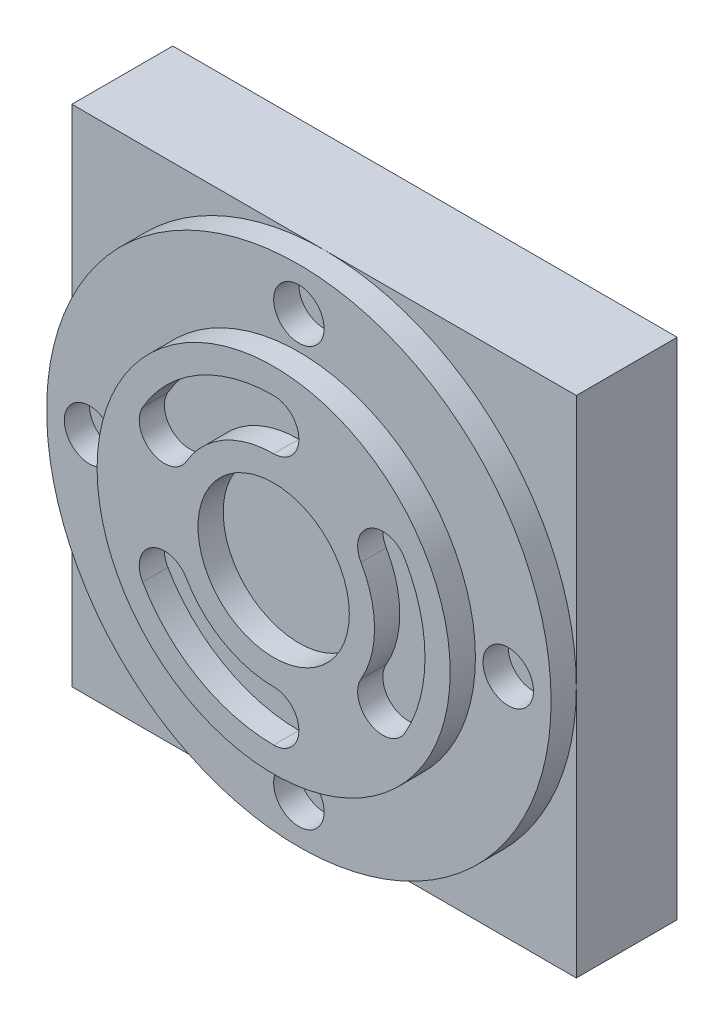
ISO-10303-21;
HEADER;
FILE_DESCRIPTION(('STEP AP214'),'2;1');
FILE_NAME('part.step','',(''),(''),'','','');
FILE_SCHEMA(('AUTOMOTIVE_DESIGN { 1 0 10303 214 1 1 1 1 }'));
ENDSEC;
DATA;
#1=APPLICATION_CONTEXT('core data for automotive mechanical design processes');
#2=APPLICATION_PROTOCOL_DEFINITION('international standard','automotive_design',2000,#1);
#3=PRODUCT_CONTEXT('',#1,'mechanical');
#4=PRODUCT('Part','Part','',(#3));
#5=PRODUCT_RELATED_PRODUCT_CATEGORY('part','',(#4));
#6=PRODUCT_DEFINITION_FORMATION('','',#4);
#7=PRODUCT_DEFINITION_CONTEXT('part definition',#1,'design');
#8=PRODUCT_DEFINITION('design','',#6,#7);
#9=PRODUCT_DEFINITION_SHAPE('','',#8);
#10=(LENGTH_UNIT() NAMED_UNIT(*) SI_UNIT(.MILLI.,.METRE.));
#11=(NAMED_UNIT(*) PLANE_ANGLE_UNIT() SI_UNIT($,.RADIAN.));
#12=(NAMED_UNIT(*) SI_UNIT($,.STERADIAN.) SOLID_ANGLE_UNIT());
#13=UNCERTAINTY_MEASURE_WITH_UNIT(LENGTH_MEASURE(1.E-05),#10,'distance_accuracy_value','');
#14=(GEOMETRIC_REPRESENTATION_CONTEXT(3) GLOBAL_UNCERTAINTY_ASSIGNED_CONTEXT((#13)) GLOBAL_UNIT_ASSIGNED_CONTEXT((#10,
#11,#12)) REPRESENTATION_CONTEXT('',''));
#15=CARTESIAN_POINT('',(0.,0.,0.));
#16=DIRECTION('',(0.,0.,1.));
#17=DIRECTION('',(1.,0.,0.));
#18=AXIS2_PLACEMENT_3D('',#15,#16,#17);
#19=CARTESIAN_POINT('',(0.,0.,20.));
#20=DIRECTION('',(0.,0.,1.));
#21=DIRECTION('',(1.,0.,0.));
#22=AXIS2_PLACEMENT_3D('',#19,#20,#21);
#23=PLANE('',#22);
#24=CARTESIAN_POINT('',(50.,50.,20.));
#25=DIRECTION('',(0.,0.,1.));
#26=DIRECTION('',(1.,0.,0.));
#27=AXIS2_PLACEMENT_3D('',#24,#25,#26);
#28=CIRCLE('',#27,50.);
#29=CARTESIAN_POINT('',(100.,50.,20.));
#30=VERTEX_POINT('',#29);
#31=CARTESIAN_POINT('',(50.,100.,20.));
#32=VERTEX_POINT('',#31);
#33=EDGE_CURVE('E49',#30,#32,#28,.T.);
#34=ORIENTED_EDGE('',*,*,#33,.F.);
#35=DIRECTION('',(0.,1.,0.));
#36=VECTOR('',#35,1.);
#37=CARTESIAN_POINT('',(100.,0.,20.));
#38=LINE('',#37,#36);
#39=CARTESIAN_POINT('',(100.,100.,20.));
#40=VERTEX_POINT('',#39);
#41=EDGE_CURVE('E320',#30,#40,#38,.T.);
#42=ORIENTED_EDGE('',*,*,#41,.T.);
#43=DIRECTION('',(-1.,0.,0.));
#44=VECTOR('',#43,1.);
#45=CARTESIAN_POINT('',(100.,100.,20.));
#46=LINE('',#45,#44);
#47=EDGE_CURVE('E321',#40,#32,#46,.T.);
#48=ORIENTED_EDGE('',*,*,#47,.T.);
#49=EDGE_LOOP('',(#34,#42,#48));
#50=FACE_BOUND('',#49,.T.);
#51=ADVANCED_FACE('F39',(#50),#23,.T.);
#52=CARTESIAN_POINT('',(0.,50.,20.));
#53=VERTEX_POINT('',#52);
#54=EDGE_CURVE('E11',#32,#53,#28,.T.);
#55=ORIENTED_EDGE('',*,*,#54,.F.);
#56=CARTESIAN_POINT('',(0.,100.,20.));
#57=VERTEX_POINT('',#56);
#58=EDGE_CURVE('E319',#32,#57,#46,.T.);
#59=ORIENTED_EDGE('',*,*,#58,.T.);
#60=DIRECTION('',(0.,-1.,0.));
#61=VECTOR('',#60,1.);
#62=CARTESIAN_POINT('',(0.,100.,20.));
#63=LINE('',#62,#61);
#64=EDGE_CURVE('E310',#57,#53,#63,.T.);
#65=ORIENTED_EDGE('',*,*,#64,.T.);
#66=EDGE_LOOP('',(#55,#59,#65));
#67=FACE_BOUND('',#66,.T.);
#68=ADVANCED_FACE('F360',(#67),#23,.T.);
#69=CARTESIAN_POINT('',(50.,0.,20.));
#70=VERTEX_POINT('',#69);
#71=EDGE_CURVE('E48',#53,#70,#28,.T.);
#72=ORIENTED_EDGE('',*,*,#71,.F.);
#73=CARTESIAN_POINT('',(0.,0.,20.));
#74=VERTEX_POINT('',#73);
#75=EDGE_CURVE('E311',#53,#74,#63,.T.);
#76=ORIENTED_EDGE('',*,*,#75,.T.);
#77=DIRECTION('',(1.,0.,0.));
#78=VECTOR('',#77,1.);
#79=CARTESIAN_POINT('',(0.,0.,20.));
#80=LINE('',#79,#78);
#81=EDGE_CURVE('E314',#74,#70,#80,.T.);
#82=ORIENTED_EDGE('',*,*,#81,.T.);
#83=EDGE_LOOP('',(#72,#76,#82));
#84=FACE_BOUND('',#83,.T.);
#85=ADVANCED_FACE('F355',(#84),#23,.T.);
#86=CARTESIAN_POINT('',(0.,100.,20.));
#87=DIRECTION('',(1.,0.,0.));
#88=DIRECTION('',(0.,0.,-1.));
#89=AXIS2_PLACEMENT_3D('',#86,#87,#88);
#90=PLANE('',#89);
#91=DIRECTION('',(0.,-1.,0.));
#92=VECTOR('',#91,1.);
#93=CARTESIAN_POINT('',(0.,100.,0.));
#94=LINE('',#93,#92);
#95=CARTESIAN_POINT('',(0.,100.,0.));
#96=VERTEX_POINT('',#95);
#97=CARTESIAN_POINT('',(0.,0.,0.));
#98=VERTEX_POINT('',#97);
#99=EDGE_CURVE('E304',#96,#98,#94,.T.);
#100=ORIENTED_EDGE('',*,*,#99,.T.);
#101=DIRECTION('',(0.,0.,-1.));
#102=VECTOR('',#101,1.);
#103=CARTESIAN_POINT('',(0.,0.,20.));
#104=LINE('',#103,#102);
#105=EDGE_CURVE('E43',#74,#98,#104,.T.);
#106=ORIENTED_EDGE('',*,*,#105,.F.);
#107=ORIENTED_EDGE('',*,*,#75,.F.);
#108=ORIENTED_EDGE('',*,*,#64,.F.);
#109=DIRECTION('',(0.,0.,-1.));
#110=VECTOR('',#109,1.);
#111=CARTESIAN_POINT('',(0.,100.,20.));
#112=LINE('',#111,#110);
#113=EDGE_CURVE('E322',#57,#96,#112,.T.);
#114=ORIENTED_EDGE('',*,*,#113,.T.);
#115=EDGE_LOOP('',(#100,#106,#107,#108,#114));
#116=FACE_BOUND('',#115,.T.);
#117=ADVANCED_FACE('F41',(#116),#90,.F.);
#118=CARTESIAN_POINT('',(0.,0.,20.));
#119=DIRECTION('',(0.,1.,0.));
#120=DIRECTION('',(0.,0.,1.));
#121=AXIS2_PLACEMENT_3D('',#118,#119,#120);
#122=PLANE('',#121);
#123=DIRECTION('',(1.,0.,0.));
#124=VECTOR('',#123,1.);
#125=CARTESIAN_POINT('',(0.,0.,0.));
#126=LINE('',#125,#124);
#127=CARTESIAN_POINT('',(100.,0.,0.));
#128=VERTEX_POINT('',#127);
#129=EDGE_CURVE('E330',#98,#128,#126,.T.);
#130=ORIENTED_EDGE('',*,*,#129,.T.);
#131=DIRECTION('',(0.,0.,-1.));
#132=VECTOR('',#131,1.);
#133=CARTESIAN_POINT('',(100.,0.,20.));
#134=LINE('',#133,#132);
#135=CARTESIAN_POINT('',(100.,0.,20.));
#136=VERTEX_POINT('',#135);
#137=EDGE_CURVE('E339',#136,#128,#134,.T.);
#138=ORIENTED_EDGE('',*,*,#137,.F.);
#139=EDGE_CURVE('E315',#70,#136,#80,.T.);
#140=ORIENTED_EDGE('',*,*,#139,.F.);
#141=ORIENTED_EDGE('',*,*,#81,.F.);
#142=ORIENTED_EDGE('',*,*,#105,.T.);
#143=EDGE_LOOP('',(#130,#138,#140,#141,#142));
#144=FACE_BOUND('',#143,.T.);
#145=ADVANCED_FACE('F370',(#144),#122,.F.);
#146=CARTESIAN_POINT('',(100.,0.,20.));
#147=DIRECTION('',(-1.,0.,0.));
#148=DIRECTION('',(0.,0.,1.));
#149=AXIS2_PLACEMENT_3D('',#146,#147,#148);
#150=PLANE('',#149);
#151=DIRECTION('',(0.,1.,0.));
#152=VECTOR('',#151,1.);
#153=CARTESIAN_POINT('',(100.,0.,0.));
#154=LINE('',#153,#152);
#155=CARTESIAN_POINT('',(100.,100.,0.));
#156=VERTEX_POINT('',#155);
#157=EDGE_CURVE('E328',#128,#156,#154,.T.);
#158=ORIENTED_EDGE('',*,*,#157,.T.);
#159=DIRECTION('',(0.,0.,-1.));
#160=VECTOR('',#159,1.);
#161=CARTESIAN_POINT('',(100.,100.,20.));
#162=LINE('',#161,#160);
#163=EDGE_CURVE('E333',#40,#156,#162,.T.);
#164=ORIENTED_EDGE('',*,*,#163,.F.);
#165=ORIENTED_EDGE('',*,*,#41,.F.);
#166=EDGE_CURVE('E318',#136,#30,#38,.T.);
#167=ORIENTED_EDGE('',*,*,#166,.F.);
#168=ORIENTED_EDGE('',*,*,#137,.T.);
#169=EDGE_LOOP('',(#158,#164,#165,#167,#168));
#170=FACE_BOUND('',#169,.T.);
#171=ADVANCED_FACE('F367',(#170),#150,.F.);
#172=CARTESIAN_POINT('',(100.,100.,20.));
#173=DIRECTION('',(0.,-1.,0.));
#174=DIRECTION('',(0.,0.,-1.));
#175=AXIS2_PLACEMENT_3D('',#172,#173,#174);
#176=PLANE('',#175);
#177=DIRECTION('',(-1.,0.,0.));
#178=VECTOR('',#177,1.);
#179=CARTESIAN_POINT('',(100.,100.,0.));
#180=LINE('',#179,#178);
#181=EDGE_CURVE('E332',#156,#96,#180,.T.);
#182=ORIENTED_EDGE('',*,*,#181,.T.);
#183=ORIENTED_EDGE('',*,*,#113,.F.);
#184=ORIENTED_EDGE('',*,*,#58,.F.);
#185=ORIENTED_EDGE('',*,*,#47,.F.);
#186=ORIENTED_EDGE('',*,*,#163,.T.);
#187=EDGE_LOOP('',(#182,#183,#184,#185,#186));
#188=FACE_BOUND('',#187,.T.);
#189=ADVANCED_FACE('F362',(#188),#176,.F.);
#190=EDGE_CURVE('E306',#70,#30,#28,.T.);
#191=ORIENTED_EDGE('',*,*,#190,.F.);
#192=ORIENTED_EDGE('',*,*,#139,.T.);
#193=ORIENTED_EDGE('',*,*,#166,.T.);
#194=EDGE_LOOP('',(#191,#192,#193));
#195=FACE_BOUND('',#194,.T.);
#196=ADVANCED_FACE('F372',(#195),#23,.T.);
#197=CARTESIAN_POINT('',(0.,0.,0.));
#198=DIRECTION('',(0.,0.,1.));
#199=DIRECTION('',(1.,0.,0.));
#200=AXIS2_PLACEMENT_3D('',#197,#198,#199);
#201=PLANE('',#200);
#202=ORIENTED_EDGE('',*,*,#99,.F.);
#203=ORIENTED_EDGE('',*,*,#181,.F.);
#204=ORIENTED_EDGE('',*,*,#157,.F.);
#205=ORIENTED_EDGE('',*,*,#129,.F.);
#206=EDGE_LOOP('',(#202,#203,#204,#205));
#207=FACE_BOUND('',#206,.T.);
#208=ADVANCED_FACE('F368',(#207),#201,.F.);
#209=CARTESIAN_POINT('',(50.,50.,25.));
#210=DIRECTION('',(0.,0.,-1.));
#211=DIRECTION('',(-1.,0.,0.));
#212=AXIS2_PLACEMENT_3D('',#209,#210,#211);
#213=CYLINDRICAL_SURFACE('',#212,50.);
#214=CARTESIAN_POINT('',(50.,50.,25.));
#215=DIRECTION('',(0.,0.,1.));
#216=DIRECTION('',(1.,0.,0.));
#217=AXIS2_PLACEMENT_3D('',#214,#215,#216);
#218=CIRCLE('',#217,50.);
#219=CARTESIAN_POINT('',(100.,50.,25.));
#220=VERTEX_POINT('',#219);
#221=EDGE_CURVE('E302',#220,#220,#218,.T.);
#222=ORIENTED_EDGE('',*,*,#221,.F.);
#223=EDGE_LOOP('',(#222));
#224=FACE_BOUND('',#223,.T.);
#225=ORIENTED_EDGE('',*,*,#33,.T.);
#226=ORIENTED_EDGE('',*,*,#54,.T.);
#227=ORIENTED_EDGE('',*,*,#71,.T.);
#228=ORIENTED_EDGE('',*,*,#190,.T.);
#229=EDGE_LOOP('',(#225,#226,#227,#228));
#230=FACE_BOUND('',#229,.T.);
#231=ADVANCED_FACE('F348',(#224,#230),#213,.T.);
#232=CARTESIAN_POINT('',(50.,50.,25.));
#233=DIRECTION('',(0.,0.,1.));
#234=DIRECTION('',(1.,0.,0.));
#235=AXIS2_PLACEMENT_3D('',#232,#233,#234);
#236=PLANE('',#235);
#237=CARTESIAN_POINT('',(50.,50.,25.));
#238=DIRECTION('',(0.,0.,1.));
#239=DIRECTION('',(1.,0.,0.));
#240=AXIS2_PLACEMENT_3D('',#237,#238,#239);
#241=CIRCLE('',#240,35.);
#242=CARTESIAN_POINT('',(85.,50.,25.));
#243=VERTEX_POINT('',#242);
#244=EDGE_CURVE('E270',#243,#243,#241,.T.);
#245=ORIENTED_EDGE('',*,*,#244,.F.);
#246=EDGE_LOOP('',(#245));
#247=FACE_BOUND('',#246,.T.);
#248=CARTESIAN_POINT('',(50.,91.5,25.));
#249=DIRECTION('',(0.,0.,1.));
#250=DIRECTION('',(1.,0.,0.));
#251=AXIS2_PLACEMENT_3D('',#248,#249,#250);
#252=CIRCLE('',#251,5.);
#253=CARTESIAN_POINT('',(55.,91.5,25.));
#254=VERTEX_POINT('',#253);
#255=EDGE_CURVE('E285',#254,#254,#252,.T.);
#256=ORIENTED_EDGE('',*,*,#255,.F.);
#257=EDGE_LOOP('',(#256));
#258=FACE_BOUND('',#257,.T.);
#259=CARTESIAN_POINT('',(91.5000000000006,50.0000000000004,25.));
#260=DIRECTION('',(0.,0.,1.));
#261=DIRECTION('',(1.,0.,0.));
#262=AXIS2_PLACEMENT_3D('',#259,#260,#261);
#263=CIRCLE('',#262,5.);
#264=CARTESIAN_POINT('',(96.5000000000006,50.0000000000004,25.));
#265=VERTEX_POINT('',#264);
#266=EDGE_CURVE('E288',#265,#265,#263,.T.);
#267=ORIENTED_EDGE('',*,*,#266,.F.);
#268=EDGE_LOOP('',(#267));
#269=FACE_BOUND('',#268,.T.);
#270=CARTESIAN_POINT('',(50.0000000000009,8.50000000000001,25.));
#271=DIRECTION('',(0.,0.,1.));
#272=DIRECTION('',(1.,0.,0.));
#273=AXIS2_PLACEMENT_3D('',#270,#271,#272);
#274=CIRCLE('',#273,5.);
#275=CARTESIAN_POINT('',(55.0000000000009,8.50000000000001,25.));
#276=VERTEX_POINT('',#275);
#277=EDGE_CURVE('E293',#276,#276,#274,.T.);
#278=ORIENTED_EDGE('',*,*,#277,.F.);
#279=EDGE_LOOP('',(#278));
#280=FACE_BOUND('',#279,.T.);
#281=CARTESIAN_POINT('',(8.50000000000059,49.9999999999999,25.));
#282=DIRECTION('',(0.,0.,1.));
#283=DIRECTION('',(1.,0.,0.));
#284=AXIS2_PLACEMENT_3D('',#281,#282,#283);
#285=CIRCLE('',#284,5.);
#286=CARTESIAN_POINT('',(13.5000000000006,49.9999999999999,25.));
#287=VERTEX_POINT('',#286);
#288=EDGE_CURVE('E280',#287,#287,#285,.T.);
#289=ORIENTED_EDGE('',*,*,#288,.F.);
#290=EDGE_LOOP('',(#289));
#291=FACE_BOUND('',#290,.T.);
#292=ORIENTED_EDGE('',*,*,#221,.T.);
#293=EDGE_LOOP('',(#292));
#294=FACE_BOUND('',#293,.T.);
#295=ADVANCED_FACE('F446',(#247,#258,#269,#280,#291,#294),#236,.T.);
#296=CARTESIAN_POINT('',(8.50000000000059,49.9999999999999,20.));
#297=DIRECTION('',(0.,0.,1.));
#298=DIRECTION('',(1.,0.,0.));
#299=AXIS2_PLACEMENT_3D('',#296,#297,#298);
#300=CYLINDRICAL_SURFACE('',#299,5.);
#301=CARTESIAN_POINT('',(8.50000000000059,49.9999999999999,20.));
#302=DIRECTION('',(0.,0.,1.));
#303=DIRECTION('',(1.,0.,0.));
#304=AXIS2_PLACEMENT_3D('',#301,#302,#303);
#305=CIRCLE('',#304,5.);
#306=CARTESIAN_POINT('',(13.5000000000006,49.9999999999999,20.));
#307=VERTEX_POINT('',#306);
#308=EDGE_CURVE('E300',#307,#307,#305,.T.);
#309=ORIENTED_EDGE('',*,*,#308,.F.);
#310=EDGE_LOOP('',(#309));
#311=FACE_BOUND('',#310,.T.);
#312=ORIENTED_EDGE('',*,*,#288,.T.);
#313=EDGE_LOOP('',(#312));
#314=FACE_BOUND('',#313,.T.);
#315=ADVANCED_FACE('F460',(#311,#314),#300,.F.);
#316=CARTESIAN_POINT('',(8.50000000000059,49.9999999999999,20.));
#317=DIRECTION('',(0.,0.,1.));
#318=DIRECTION('',(1.,0.,0.));
#319=AXIS2_PLACEMENT_3D('',#316,#317,#318);
#320=PLANE('',#319);
#321=ORIENTED_EDGE('',*,*,#308,.T.);
#322=EDGE_LOOP('',(#321));
#323=FACE_BOUND('',#322,.T.);
#324=ADVANCED_FACE('F466',(#323),#320,.T.);
#325=CARTESIAN_POINT('',(50.0000000000009,8.50000000000001,20.));
#326=DIRECTION('',(0.,0.,1.));
#327=DIRECTION('',(1.,0.,0.));
#328=AXIS2_PLACEMENT_3D('',#325,#326,#327);
#329=CYLINDRICAL_SURFACE('',#328,5.);
#330=CARTESIAN_POINT('',(50.0000000000009,8.50000000000001,20.));
#331=DIRECTION('',(0.,0.,1.));
#332=DIRECTION('',(1.,0.,0.));
#333=AXIS2_PLACEMENT_3D('',#330,#331,#332);
#334=CIRCLE('',#333,5.);
#335=CARTESIAN_POINT('',(55.0000000000009,8.50000000000001,20.));
#336=VERTEX_POINT('',#335);
#337=EDGE_CURVE('E295',#336,#336,#334,.T.);
#338=ORIENTED_EDGE('',*,*,#337,.F.);
#339=EDGE_LOOP('',(#338));
#340=FACE_BOUND('',#339,.T.);
#341=ORIENTED_EDGE('',*,*,#277,.T.);
#342=EDGE_LOOP('',(#341));
#343=FACE_BOUND('',#342,.T.);
#344=ADVANCED_FACE('F474',(#340,#343),#329,.F.);
#345=CARTESIAN_POINT('',(50.0000000000009,8.50000000000001,20.));
#346=DIRECTION('',(0.,0.,1.));
#347=DIRECTION('',(1.,0.,0.));
#348=AXIS2_PLACEMENT_3D('',#345,#346,#347);
#349=PLANE('',#348);
#350=ORIENTED_EDGE('',*,*,#337,.T.);
#351=EDGE_LOOP('',(#350));
#352=FACE_BOUND('',#351,.T.);
#353=ADVANCED_FACE('F482',(#352),#349,.T.);
#354=CARTESIAN_POINT('',(91.5000000000006,50.0000000000004,20.));
#355=DIRECTION('',(0.,0.,1.));
#356=DIRECTION('',(1.,0.,0.));
#357=AXIS2_PLACEMENT_3D('',#354,#355,#356);
#358=CYLINDRICAL_SURFACE('',#357,5.);
#359=CARTESIAN_POINT('',(91.5000000000006,50.0000000000004,20.));
#360=DIRECTION('',(0.,0.,1.));
#361=DIRECTION('',(1.,0.,0.));
#362=AXIS2_PLACEMENT_3D('',#359,#360,#361);
#363=CIRCLE('',#362,5.);
#364=CARTESIAN_POINT('',(96.5000000000006,50.0000000000004,20.));
#365=VERTEX_POINT('',#364);
#366=EDGE_CURVE('E286',#365,#365,#363,.T.);
#367=ORIENTED_EDGE('',*,*,#366,.F.);
#368=EDGE_LOOP('',(#367));
#369=FACE_BOUND('',#368,.T.);
#370=ORIENTED_EDGE('',*,*,#266,.T.);
#371=EDGE_LOOP('',(#370));
#372=FACE_BOUND('',#371,.T.);
#373=ADVANCED_FACE('F492',(#369,#372),#358,.F.);
#374=CARTESIAN_POINT('',(91.5000000000006,50.0000000000004,20.));
#375=DIRECTION('',(0.,0.,1.));
#376=DIRECTION('',(1.,0.,0.));
#377=AXIS2_PLACEMENT_3D('',#374,#375,#376);
#378=PLANE('',#377);
#379=ORIENTED_EDGE('',*,*,#366,.T.);
#380=EDGE_LOOP('',(#379));
#381=FACE_BOUND('',#380,.T.);
#382=ADVANCED_FACE('F504',(#381),#378,.T.);
#383=CARTESIAN_POINT('',(50.,91.5,20.));
#384=DIRECTION('',(0.,0.,1.));
#385=DIRECTION('',(1.,0.,0.));
#386=AXIS2_PLACEMENT_3D('',#383,#384,#385);
#387=CYLINDRICAL_SURFACE('',#386,5.);
#388=CARTESIAN_POINT('',(50.,91.5,20.));
#389=DIRECTION('',(0.,0.,1.));
#390=DIRECTION('',(1.,0.,0.));
#391=AXIS2_PLACEMENT_3D('',#388,#389,#390);
#392=CIRCLE('',#391,5.);
#393=CARTESIAN_POINT('',(55.,91.5,20.));
#394=VERTEX_POINT('',#393);
#395=EDGE_CURVE('E278',#394,#394,#392,.T.);
#396=ORIENTED_EDGE('',*,*,#395,.F.);
#397=EDGE_LOOP('',(#396));
#398=FACE_BOUND('',#397,.T.);
#399=ORIENTED_EDGE('',*,*,#255,.T.);
#400=EDGE_LOOP('',(#399));
#401=FACE_BOUND('',#400,.T.);
#402=ADVANCED_FACE('F512',(#398,#401),#387,.F.);
#403=CARTESIAN_POINT('',(50.,91.5,20.));
#404=DIRECTION('',(0.,0.,1.));
#405=DIRECTION('',(1.,0.,0.));
#406=AXIS2_PLACEMENT_3D('',#403,#404,#405);
#407=PLANE('',#406);
#408=ORIENTED_EDGE('',*,*,#395,.T.);
#409=EDGE_LOOP('',(#408));
#410=FACE_BOUND('',#409,.T.);
#411=ADVANCED_FACE('F518',(#410),#407,.T.);
#412=CARTESIAN_POINT('',(50.,50.,30.));
#413=DIRECTION('',(0.,0.,-1.));
#414=DIRECTION('',(-1.,0.,0.));
#415=AXIS2_PLACEMENT_3D('',#412,#413,#414);
#416=CYLINDRICAL_SURFACE('',#415,35.);
#417=CARTESIAN_POINT('',(50.,50.,30.));
#418=DIRECTION('',(0.,0.,1.));
#419=DIRECTION('',(1.,0.,0.));
#420=AXIS2_PLACEMENT_3D('',#417,#418,#419);
#421=CIRCLE('',#420,35.);
#422=CARTESIAN_POINT('',(85.,50.,30.));
#423=VERTEX_POINT('',#422);
#424=EDGE_CURVE('E273',#423,#423,#421,.T.);
#425=ORIENTED_EDGE('',*,*,#424,.F.);
#426=EDGE_LOOP('',(#425));
#427=FACE_BOUND('',#426,.T.);
#428=ORIENTED_EDGE('',*,*,#244,.T.);
#429=EDGE_LOOP('',(#428));
#430=FACE_BOUND('',#429,.T.);
#431=ADVANCED_FACE('F530',(#427,#430),#416,.T.);
#432=CARTESIAN_POINT('',(50.,50.,30.));
#433=DIRECTION('',(0.,0.,1.));
#434=DIRECTION('',(1.,0.,0.));
#435=AXIS2_PLACEMENT_3D('',#432,#433,#434);
#436=PLANE('',#435);
#437=CARTESIAN_POINT('',(71.6506350946109,37.4999999999999,30.));
#438=DIRECTION('',(0.,0.,1.));
#439=DIRECTION('',(-0.500000000000004,-0.866025403784436,0.));
#440=AXIS2_PLACEMENT_3D('',#437,#438,#439);
#441=CIRCLE('',#440,4.99999999999999);
#442=CARTESIAN_POINT('',(67.3205080756888,39.9999999999999,30.));
#443=VERTEX_POINT('',#442);
#444=CARTESIAN_POINT('',(75.9807621135331,34.9999999999999,30.));
#445=VERTEX_POINT('',#444);
#446=EDGE_CURVE('E60',#443,#445,#441,.T.);
#447=ORIENTED_EDGE('',*,*,#446,.F.);
#448=CARTESIAN_POINT('',(50.,50.,30.));
#449=DIRECTION('',(0.,0.,-1.));
#450=DIRECTION('',(-0.500000000000004,-0.866025403784436,0.));
#451=AXIS2_PLACEMENT_3D('',#448,#449,#450);
#452=CIRCLE('',#451,20.);
#453=CARTESIAN_POINT('',(67.3205080756888,60.,30.));
#454=VERTEX_POINT('',#453);
#455=EDGE_CURVE('E189',#454,#443,#452,.T.);
#456=ORIENTED_EDGE('',*,*,#455,.F.);
#457=CARTESIAN_POINT('',(71.6506350946109,62.5000000000002,30.));
#458=DIRECTION('',(0.,0.,1.));
#459=DIRECTION('',(-0.500000000000004,-0.866025403784436,0.));
#460=AXIS2_PLACEMENT_3D('',#457,#458,#459);
#461=CIRCLE('',#460,4.99999999999999);
#462=CARTESIAN_POINT('',(75.980762113533,65.0000000000003,30.));
#463=VERTEX_POINT('',#462);
#464=EDGE_CURVE('E188',#463,#454,#461,.T.);
#465=ORIENTED_EDGE('',*,*,#464,.F.);
#466=CARTESIAN_POINT('',(50.,50.,30.));
#467=DIRECTION('',(0.,0.,1.));
#468=DIRECTION('',(-0.500000000000004,-0.866025403784436,0.));
#469=AXIS2_PLACEMENT_3D('',#466,#467,#468);
#470=CIRCLE('',#469,30.);
#471=EDGE_CURVE('E198',#445,#463,#470,.T.);
#472=ORIENTED_EDGE('',*,*,#471,.F.);
#473=EDGE_LOOP('',(#447,#456,#465,#472));
#474=FACE_BOUND('',#473,.T.);
#475=CARTESIAN_POINT('',(28.3493649053889,37.5000000000002,30.));
#476=DIRECTION('',(0.,0.,1.));
#477=DIRECTION('',(-0.499999999999992,0.866025403784443,0.));
#478=AXIS2_PLACEMENT_3D('',#475,#476,#477);
#479=CIRCLE('',#478,4.99999999999999);
#480=CARTESIAN_POINT('',(32.6794919243111,40.0000000000001,30.));
#481=VERTEX_POINT('',#480);
#482=CARTESIAN_POINT('',(24.0192378864667,35.0000000000002,30.));
#483=VERTEX_POINT('',#482);
#484=EDGE_CURVE('E63',#481,#483,#479,.T.);
#485=ORIENTED_EDGE('',*,*,#484,.F.);
#486=CARTESIAN_POINT('',(50.,50.,30.));
#487=DIRECTION('',(0.,0.,-1.));
#488=DIRECTION('',(-0.499999999999992,0.866025403784443,0.));
#489=AXIS2_PLACEMENT_3D('',#486,#487,#488);
#490=CIRCLE('',#489,20.);
#491=CARTESIAN_POINT('',(49.9999999999999,30.,30.));
#492=VERTEX_POINT('',#491);
#493=EDGE_CURVE('E211',#492,#481,#490,.T.);
#494=ORIENTED_EDGE('',*,*,#493,.F.);
#495=CARTESIAN_POINT('',(50.0000000000001,25.,30.));
#496=DIRECTION('',(0.,0.,1.));
#497=DIRECTION('',(-0.499999999999992,0.866025403784443,0.));
#498=AXIS2_PLACEMENT_3D('',#495,#496,#497);
#499=CIRCLE('',#498,4.99999999999999);
#500=CARTESIAN_POINT('',(50.0000000000001,20.,30.));
#501=VERTEX_POINT('',#500);
#502=EDGE_CURVE('E223',#501,#492,#499,.T.);
#503=ORIENTED_EDGE('',*,*,#502,.F.);
#504=CARTESIAN_POINT('',(50.,50.,30.));
#505=DIRECTION('',(0.,0.,1.));
#506=DIRECTION('',(-0.499999999999992,0.866025403784443,0.));
#507=AXIS2_PLACEMENT_3D('',#504,#505,#506);
#508=CIRCLE('',#507,30.);
#509=EDGE_CURVE('E225',#483,#501,#508,.T.);
#510=ORIENTED_EDGE('',*,*,#509,.F.);
#511=EDGE_LOOP('',(#485,#494,#503,#510));
#512=FACE_BOUND('',#511,.T.);
#513=CARTESIAN_POINT('',(50.,50.,30.));
#514=DIRECTION('',(0.,0.,1.));
#515=DIRECTION('',(1.,0.,0.));
#516=AXIS2_PLACEMENT_3D('',#513,#514,#515);
#517=CIRCLE('',#516,15.);
#518=CARTESIAN_POINT('',(65.,50.,30.));
#519=VERTEX_POINT('',#518);
#520=EDGE_CURVE('E201',#519,#519,#517,.T.);
#521=ORIENTED_EDGE('',*,*,#520,.F.);
#522=EDGE_LOOP('',(#521));
#523=FACE_BOUND('',#522,.T.);
#524=CARTESIAN_POINT('',(50.,75.,30.));
#525=DIRECTION('',(0.,0.,1.));
#526=DIRECTION('',(1.,0.,0.));
#527=AXIS2_PLACEMENT_3D('',#524,#525,#526);
#528=CIRCLE('',#527,4.99999999999999);
#529=CARTESIAN_POINT('',(50.,70.,30.));
#530=VERTEX_POINT('',#529);
#531=CARTESIAN_POINT('',(50.,80.,30.));
#532=VERTEX_POINT('',#531);
#533=EDGE_CURVE('E239',#530,#532,#528,.T.);
#534=ORIENTED_EDGE('',*,*,#533,.F.);
#535=CARTESIAN_POINT('',(50.,50.,30.));
#536=DIRECTION('',(0.,0.,-1.));
#537=DIRECTION('',(1.,0.,0.));
#538=AXIS2_PLACEMENT_3D('',#535,#536,#537);
#539=CIRCLE('',#538,20.);
#540=CARTESIAN_POINT('',(32.6794919243112,60.,30.));
#541=VERTEX_POINT('',#540);
#542=EDGE_CURVE('E246',#541,#530,#539,.T.);
#543=ORIENTED_EDGE('',*,*,#542,.F.);
#544=CARTESIAN_POINT('',(28.3493649053889,62.4999999999997,30.));
#545=DIRECTION('',(0.,0.,1.));
#546=DIRECTION('',(1.,0.,0.));
#547=AXIS2_PLACEMENT_3D('',#544,#545,#546);
#548=CIRCLE('',#547,4.99999999999999);
#549=CARTESIAN_POINT('',(24.0192378864666,64.9999999999997,30.));
#550=VERTEX_POINT('',#549);
#551=EDGE_CURVE('E257',#550,#541,#548,.T.);
#552=ORIENTED_EDGE('',*,*,#551,.F.);
#553=CARTESIAN_POINT('',(50.,50.,30.));
#554=DIRECTION('',(0.,0.,1.));
#555=DIRECTION('',(1.,0.,0.));
#556=AXIS2_PLACEMENT_3D('',#553,#554,#555);
#557=CIRCLE('',#556,30.);
#558=EDGE_CURVE('E260',#532,#550,#557,.T.);
#559=ORIENTED_EDGE('',*,*,#558,.F.);
#560=EDGE_LOOP('',(#534,#543,#552,#559));
#561=FACE_BOUND('',#560,.T.);
#562=ORIENTED_EDGE('',*,*,#424,.T.);
#563=EDGE_LOOP('',(#562));
#564=FACE_BOUND('',#563,.T.);
#565=ADVANCED_FACE('F538',(#474,#512,#523,#561,#564),#436,.T.);
#566=CARTESIAN_POINT('',(50.,75.,25.));
#567=DIRECTION('',(0.,0.,1.));
#568=DIRECTION('',(1.,0.,0.));
#569=AXIS2_PLACEMENT_3D('',#566,#567,#568);
#570=CYLINDRICAL_SURFACE('',#569,4.99999999999999);
#571=ORIENTED_EDGE('',*,*,#533,.T.);
#572=DIRECTION('',(0.,0.,1.));
#573=VECTOR('',#572,1.);
#574=CARTESIAN_POINT('',(50.,80.,25.));
#575=LINE('',#574,#573);
#576=CARTESIAN_POINT('',(50.,80.,25.));
#577=VERTEX_POINT('',#576);
#578=EDGE_CURVE('E254',#577,#532,#575,.T.);
#579=ORIENTED_EDGE('',*,*,#578,.F.);
#580=CARTESIAN_POINT('',(50.,75.,25.));
#581=DIRECTION('',(0.,0.,1.));
#582=DIRECTION('',(1.,0.,0.));
#583=AXIS2_PLACEMENT_3D('',#580,#581,#582);
#584=CIRCLE('',#583,4.99999999999999);
#585=CARTESIAN_POINT('',(50.,70.,25.));
#586=VERTEX_POINT('',#585);
#587=EDGE_CURVE('E244',#586,#577,#584,.T.);
#588=ORIENTED_EDGE('',*,*,#587,.F.);
#589=DIRECTION('',(0.,0.,1.));
#590=VECTOR('',#589,1.);
#591=CARTESIAN_POINT('',(50.,70.,25.));
#592=LINE('',#591,#590);
#593=EDGE_CURVE('E264',#586,#530,#592,.T.);
#594=ORIENTED_EDGE('',*,*,#593,.T.);
#595=EDGE_LOOP('',(#571,#579,#588,#594));
#596=FACE_BOUND('',#595,.T.);
#597=ADVANCED_FACE('F550',(#596),#570,.F.);
#598=CARTESIAN_POINT('',(50.,50.,25.));
#599=DIRECTION('',(0.,0.,1.));
#600=DIRECTION('',(1.,0.,0.));
#601=AXIS2_PLACEMENT_3D('',#598,#599,#600);
#602=CYLINDRICAL_SURFACE('',#601,20.);
#603=ORIENTED_EDGE('',*,*,#542,.T.);
#604=ORIENTED_EDGE('',*,*,#593,.F.);
#605=CARTESIAN_POINT('',(50.,50.,25.));
#606=DIRECTION('',(0.,0.,-1.));
#607=DIRECTION('',(1.,0.,0.));
#608=AXIS2_PLACEMENT_3D('',#605,#606,#607);
#609=CIRCLE('',#608,20.);
#610=CARTESIAN_POINT('',(32.6794919243112,60.,25.));
#611=VERTEX_POINT('',#610);
#612=EDGE_CURVE('E252',#611,#586,#609,.T.);
#613=ORIENTED_EDGE('',*,*,#612,.F.);
#614=DIRECTION('',(0.,0.,1.));
#615=VECTOR('',#614,1.);
#616=CARTESIAN_POINT('',(32.6794919243112,60.,25.));
#617=LINE('',#616,#615);
#618=EDGE_CURVE('E268',#611,#541,#617,.T.);
#619=ORIENTED_EDGE('',*,*,#618,.T.);
#620=EDGE_LOOP('',(#603,#604,#613,#619));
#621=FACE_BOUND('',#620,.T.);
#622=ADVANCED_FACE('F557',(#621),#602,.T.);
#623=CARTESIAN_POINT('',(28.3493649053889,62.4999999999997,25.));
#624=DIRECTION('',(0.,0.,1.));
#625=DIRECTION('',(1.,0.,0.));
#626=AXIS2_PLACEMENT_3D('',#623,#624,#625);
#627=CYLINDRICAL_SURFACE('',#626,4.99999999999999);
#628=ORIENTED_EDGE('',*,*,#551,.T.);
#629=ORIENTED_EDGE('',*,*,#618,.F.);
#630=CARTESIAN_POINT('',(28.3493649053889,62.4999999999997,25.));
#631=DIRECTION('',(0.,0.,1.));
#632=DIRECTION('',(1.,0.,0.));
#633=AXIS2_PLACEMENT_3D('',#630,#631,#632);
#634=CIRCLE('',#633,4.99999999999999);
#635=CARTESIAN_POINT('',(24.0192378864666,64.9999999999997,25.));
#636=VERTEX_POINT('',#635);
#637=EDGE_CURVE('E248',#636,#611,#634,.T.);
#638=ORIENTED_EDGE('',*,*,#637,.F.);
#639=DIRECTION('',(0.,0.,1.));
#640=VECTOR('',#639,1.);
#641=CARTESIAN_POINT('',(24.0192378864666,64.9999999999997,25.));
#642=LINE('',#641,#640);
#643=EDGE_CURVE('E269',#636,#550,#642,.T.);
#644=ORIENTED_EDGE('',*,*,#643,.T.);
#645=EDGE_LOOP('',(#628,#629,#638,#644));
#646=FACE_BOUND('',#645,.T.);
#647=ADVANCED_FACE('F564',(#646),#627,.F.);
#648=CARTESIAN_POINT('',(50.,50.,25.));
#649=DIRECTION('',(0.,0.,1.));
#650=DIRECTION('',(1.,0.,0.));
#651=AXIS2_PLACEMENT_3D('',#648,#649,#650);
#652=CYLINDRICAL_SURFACE('',#651,30.);
#653=ORIENTED_EDGE('',*,*,#558,.T.);
#654=ORIENTED_EDGE('',*,*,#643,.F.);
#655=CARTESIAN_POINT('',(50.,50.,25.));
#656=DIRECTION('',(0.,0.,1.));
#657=DIRECTION('',(1.,0.,0.));
#658=AXIS2_PLACEMENT_3D('',#655,#656,#657);
#659=CIRCLE('',#658,30.);
#660=EDGE_CURVE('E243',#577,#636,#659,.T.);
#661=ORIENTED_EDGE('',*,*,#660,.F.);
#662=ORIENTED_EDGE('',*,*,#578,.T.);
#663=EDGE_LOOP('',(#653,#654,#661,#662));
#664=FACE_BOUND('',#663,.T.);
#665=ADVANCED_FACE('F571',(#664),#652,.F.);
#666=CARTESIAN_POINT('',(50.,62.5,25.));
#667=DIRECTION('',(0.,0.,1.));
#668=DIRECTION('',(1.,0.,0.));
#669=AXIS2_PLACEMENT_3D('',#666,#667,#668);
#670=PLANE('',#669);
#671=ORIENTED_EDGE('',*,*,#587,.T.);
#672=ORIENTED_EDGE('',*,*,#660,.T.);
#673=ORIENTED_EDGE('',*,*,#637,.T.);
#674=ORIENTED_EDGE('',*,*,#612,.T.);
#675=EDGE_LOOP('',(#671,#672,#673,#674));
#676=FACE_BOUND('',#675,.T.);
#677=ADVANCED_FACE('F581',(#676),#670,.T.);
#678=CARTESIAN_POINT('',(50.,50.,25.));
#679=DIRECTION('',(0.,0.,1.));
#680=DIRECTION('',(1.,0.,0.));
#681=AXIS2_PLACEMENT_3D('',#678,#679,#680);
#682=CYLINDRICAL_SURFACE('',#681,15.);
#683=CARTESIAN_POINT('',(50.,50.,25.));
#684=DIRECTION('',(0.,0.,1.));
#685=DIRECTION('',(1.,0.,0.));
#686=AXIS2_PLACEMENT_3D('',#683,#684,#685);
#687=CIRCLE('',#686,15.);
#688=CARTESIAN_POINT('',(65.,50.,25.));
#689=VERTEX_POINT('',#688);
#690=EDGE_CURVE('E237',#689,#689,#687,.T.);
#691=ORIENTED_EDGE('',*,*,#690,.F.);
#692=EDGE_LOOP('',(#691));
#693=FACE_BOUND('',#692,.T.);
#694=ORIENTED_EDGE('',*,*,#520,.T.);
#695=EDGE_LOOP('',(#694));
#696=FACE_BOUND('',#695,.T.);
#697=ADVANCED_FACE('F595',(#693,#696),#682,.F.);
#698=CARTESIAN_POINT('',(50.,50.,25.));
#699=DIRECTION('',(0.,0.,1.));
#700=DIRECTION('',(1.,0.,0.));
#701=AXIS2_PLACEMENT_3D('',#698,#699,#700);
#702=PLANE('',#701);
#703=ORIENTED_EDGE('',*,*,#690,.T.);
#704=EDGE_LOOP('',(#703));
#705=FACE_BOUND('',#704,.T.);
#706=ADVANCED_FACE('F601',(#705),#702,.T.);
#707=CARTESIAN_POINT('',(28.3493649053889,37.5000000000002,25.));
#708=DIRECTION('',(0.,0.,1.));
#709=DIRECTION('',(1.,0.,0.));
#710=AXIS2_PLACEMENT_3D('',#707,#708,#709);
#711=CYLINDRICAL_SURFACE('',#710,4.99999999999999);
#712=ORIENTED_EDGE('',*,*,#484,.T.);
#713=DIRECTION('',(0.,0.,1.));
#714=VECTOR('',#713,1.);
#715=CARTESIAN_POINT('',(24.0192378864667,35.0000000000002,25.));
#716=LINE('',#715,#714);
#717=CARTESIAN_POINT('',(24.0192378864667,35.0000000000002,25.));
#718=VERTEX_POINT('',#717);
#719=EDGE_CURVE('E219',#718,#483,#716,.T.);
#720=ORIENTED_EDGE('',*,*,#719,.F.);
#721=CARTESIAN_POINT('',(28.3493649053889,37.5000000000002,25.));
#722=DIRECTION('',(0.,0.,1.));
#723=DIRECTION('',(-0.499999999999992,0.866025403784443,0.));
#724=AXIS2_PLACEMENT_3D('',#721,#722,#723);
#725=CIRCLE('',#724,4.99999999999999);
#726=CARTESIAN_POINT('',(32.6794919243111,40.0000000000001,25.));
#727=VERTEX_POINT('',#726);
#728=EDGE_CURVE('E210',#727,#718,#725,.T.);
#729=ORIENTED_EDGE('',*,*,#728,.F.);
#730=DIRECTION('',(0.,0.,1.));
#731=VECTOR('',#730,1.);
#732=CARTESIAN_POINT('',(32.6794919243111,40.0000000000001,25.));
#733=LINE('',#732,#731);
#734=EDGE_CURVE('E197',#727,#481,#733,.T.);
#735=ORIENTED_EDGE('',*,*,#734,.T.);
#736=EDGE_LOOP('',(#712,#720,#729,#735));
#737=FACE_BOUND('',#736,.T.);
#738=ADVANCED_FACE('F608',(#737),#711,.F.);
#739=CARTESIAN_POINT('',(50.,50.,25.));
#740=DIRECTION('',(0.,0.,1.));
#741=DIRECTION('',(1.,0.,0.));
#742=AXIS2_PLACEMENT_3D('',#739,#740,#741);
#743=CYLINDRICAL_SURFACE('',#742,20.);
#744=ORIENTED_EDGE('',*,*,#493,.T.);
#745=ORIENTED_EDGE('',*,*,#734,.F.);
#746=CARTESIAN_POINT('',(50.,50.,25.));
#747=DIRECTION('',(0.,0.,-1.));
#748=DIRECTION('',(-0.499999999999992,0.866025403784443,0.));
#749=AXIS2_PLACEMENT_3D('',#746,#747,#748);
#750=CIRCLE('',#749,20.);
#751=CARTESIAN_POINT('',(49.9999999999999,30.,25.));
#752=VERTEX_POINT('',#751);
#753=EDGE_CURVE('E220',#752,#727,#750,.T.);
#754=ORIENTED_EDGE('',*,*,#753,.F.);
#755=DIRECTION('',(0.,0.,1.));
#756=VECTOR('',#755,1.);
#757=CARTESIAN_POINT('',(49.9999999999999,30.,25.));
#758=LINE('',#757,#756);
#759=EDGE_CURVE('E231',#752,#492,#758,.T.);
#760=ORIENTED_EDGE('',*,*,#759,.T.);
#761=EDGE_LOOP('',(#744,#745,#754,#760));
#762=FACE_BOUND('',#761,.T.);
#763=ADVANCED_FACE('F618',(#762),#743,.T.);
#764=CARTESIAN_POINT('',(50.0000000000001,25.,25.));
#765=DIRECTION('',(0.,0.,1.));
#766=DIRECTION('',(1.,0.,0.));
#767=AXIS2_PLACEMENT_3D('',#764,#765,#766);
#768=CYLINDRICAL_SURFACE('',#767,4.99999999999999);
#769=ORIENTED_EDGE('',*,*,#502,.T.);
#770=ORIENTED_EDGE('',*,*,#759,.F.);
#771=CARTESIAN_POINT('',(50.0000000000001,25.,25.));
#772=DIRECTION('',(0.,0.,1.));
#773=DIRECTION('',(-0.499999999999992,0.866025403784443,0.));
#774=AXIS2_PLACEMENT_3D('',#771,#772,#773);
#775=CIRCLE('',#774,4.99999999999999);
#776=CARTESIAN_POINT('',(50.0000000000001,20.,25.));
#777=VERTEX_POINT('',#776);
#778=EDGE_CURVE('E212',#777,#752,#775,.T.);
#779=ORIENTED_EDGE('',*,*,#778,.F.);
#780=DIRECTION('',(0.,0.,1.));
#781=VECTOR('',#780,1.);
#782=CARTESIAN_POINT('',(50.0000000000001,20.,25.));
#783=LINE('',#782,#781);
#784=EDGE_CURVE('E232',#777,#501,#783,.T.);
#785=ORIENTED_EDGE('',*,*,#784,.T.);
#786=EDGE_LOOP('',(#769,#770,#779,#785));
#787=FACE_BOUND('',#786,.T.);
#788=ADVANCED_FACE('F629',(#787),#768,.F.);
#789=CARTESIAN_POINT('',(50.,50.,25.));
#790=DIRECTION('',(0.,0.,1.));
#791=DIRECTION('',(1.,0.,0.));
#792=AXIS2_PLACEMENT_3D('',#789,#790,#791);
#793=CYLINDRICAL_SURFACE('',#792,30.);
#794=ORIENTED_EDGE('',*,*,#509,.T.);
#795=ORIENTED_EDGE('',*,*,#784,.F.);
#796=CARTESIAN_POINT('',(50.,50.,25.));
#797=DIRECTION('',(0.,0.,1.));
#798=DIRECTION('',(-0.499999999999992,0.866025403784443,0.));
#799=AXIS2_PLACEMENT_3D('',#796,#797,#798);
#800=CIRCLE('',#799,30.);
#801=EDGE_CURVE('E209',#718,#777,#800,.T.);
#802=ORIENTED_EDGE('',*,*,#801,.F.);
#803=ORIENTED_EDGE('',*,*,#719,.T.);
#804=EDGE_LOOP('',(#794,#795,#802,#803));
#805=FACE_BOUND('',#804,.T.);
#806=ADVANCED_FACE('F638',(#805),#793,.F.);
#807=CARTESIAN_POINT('',(39.1746824526945,43.7500000000001,25.));
#808=DIRECTION('',(0.,0.,1.));
#809=DIRECTION('',(-0.499999999999992,0.866025403784443,0.));
#810=AXIS2_PLACEMENT_3D('',#807,#808,#809);
#811=PLANE('',#810);
#812=ORIENTED_EDGE('',*,*,#728,.T.);
#813=ORIENTED_EDGE('',*,*,#801,.T.);
#814=ORIENTED_EDGE('',*,*,#778,.T.);
#815=ORIENTED_EDGE('',*,*,#753,.T.);
#816=EDGE_LOOP('',(#812,#813,#814,#815));
#817=FACE_BOUND('',#816,.T.);
#818=ADVANCED_FACE('F642',(#817),#811,.T.);
#819=CARTESIAN_POINT('',(71.6506350946109,37.4999999999999,25.));
#820=DIRECTION('',(0.,0.,1.));
#821=DIRECTION('',(1.,0.,0.));
#822=AXIS2_PLACEMENT_3D('',#819,#820,#821);
#823=CYLINDRICAL_SURFACE('',#822,4.99999999999999);
#824=ORIENTED_EDGE('',*,*,#446,.T.);
#825=DIRECTION('',(0.,0.,1.));
#826=VECTOR('',#825,1.);
#827=CARTESIAN_POINT('',(75.9807621135331,34.9999999999999,25.));
#828=LINE('',#827,#826);
#829=CARTESIAN_POINT('',(75.9807621135331,34.9999999999999,25.));
#830=VERTEX_POINT('',#829);
#831=EDGE_CURVE('E164',#830,#445,#828,.T.);
#832=ORIENTED_EDGE('',*,*,#831,.F.);
#833=CARTESIAN_POINT('',(71.6506350946109,37.4999999999999,25.));
#834=DIRECTION('',(0.,0.,1.));
#835=DIRECTION('',(-0.500000000000004,-0.866025403784436,0.));
#836=AXIS2_PLACEMENT_3D('',#833,#834,#835);
#837=CIRCLE('',#836,4.99999999999999);
#838=CARTESIAN_POINT('',(67.3205080756888,39.9999999999999,25.));
#839=VERTEX_POINT('',#838);
#840=EDGE_CURVE('E166',#839,#830,#837,.T.);
#841=ORIENTED_EDGE('',*,*,#840,.F.);
#842=DIRECTION('',(0.,0.,1.));
#843=VECTOR('',#842,1.);
#844=CARTESIAN_POINT('',(67.3205080756888,39.9999999999999,25.));
#845=LINE('',#844,#843);
#846=EDGE_CURVE('E203',#839,#443,#845,.T.);
#847=ORIENTED_EDGE('',*,*,#846,.T.);
#848=EDGE_LOOP('',(#824,#832,#841,#847));
#849=FACE_BOUND('',#848,.T.);
#850=ADVANCED_FACE('F170',(#849),#823,.F.);
#851=CARTESIAN_POINT('',(50.,50.,25.));
#852=DIRECTION('',(0.,0.,1.));
#853=DIRECTION('',(1.,0.,0.));
#854=AXIS2_PLACEMENT_3D('',#851,#852,#853);
#855=CYLINDRICAL_SURFACE('',#854,20.);
#856=ORIENTED_EDGE('',*,*,#455,.T.);
#857=ORIENTED_EDGE('',*,*,#846,.F.);
#858=CARTESIAN_POINT('',(50.,50.,25.));
#859=DIRECTION('',(0.,0.,-1.));
#860=DIRECTION('',(-0.500000000000004,-0.866025403784436,0.));
#861=AXIS2_PLACEMENT_3D('',#858,#859,#860);
#862=CIRCLE('',#861,20.);
#863=CARTESIAN_POINT('',(67.3205080756888,60.,25.));
#864=VERTEX_POINT('',#863);
#865=EDGE_CURVE('E173',#864,#839,#862,.T.);
#866=ORIENTED_EDGE('',*,*,#865,.F.);
#867=DIRECTION('',(0.,0.,1.));
#868=VECTOR('',#867,1.);
#869=CARTESIAN_POINT('',(67.3205080756888,60.,25.));
#870=LINE('',#869,#868);
#871=EDGE_CURVE('E204',#864,#454,#870,.T.);
#872=ORIENTED_EDGE('',*,*,#871,.T.);
#873=EDGE_LOOP('',(#856,#857,#866,#872));
#874=FACE_BOUND('',#873,.T.);
#875=ADVANCED_FACE('F665',(#874),#855,.T.);
#876=CARTESIAN_POINT('',(71.6506350946109,62.5000000000002,25.));
#877=DIRECTION('',(0.,0.,1.));
#878=DIRECTION('',(1.,0.,0.));
#879=AXIS2_PLACEMENT_3D('',#876,#877,#878);
#880=CYLINDRICAL_SURFACE('',#879,4.99999999999999);
#881=ORIENTED_EDGE('',*,*,#464,.T.);
#882=ORIENTED_EDGE('',*,*,#871,.F.);
#883=CARTESIAN_POINT('',(71.6506350946109,62.5000000000002,25.));
#884=DIRECTION('',(0.,0.,1.));
#885=DIRECTION('',(-0.500000000000004,-0.866025403784436,0.));
#886=AXIS2_PLACEMENT_3D('',#883,#884,#885);
#887=CIRCLE('',#886,4.99999999999999);
#888=CARTESIAN_POINT('',(75.980762113533,65.0000000000003,25.));
#889=VERTEX_POINT('',#888);
#890=EDGE_CURVE('E181',#889,#864,#887,.T.);
#891=ORIENTED_EDGE('',*,*,#890,.F.);
#892=DIRECTION('',(0.,0.,1.));
#893=VECTOR('',#892,1.);
#894=CARTESIAN_POINT('',(75.980762113533,65.0000000000003,25.));
#895=LINE('',#894,#893);
#896=EDGE_CURVE('E171',#889,#463,#895,.T.);
#897=ORIENTED_EDGE('',*,*,#896,.T.);
#898=EDGE_LOOP('',(#881,#882,#891,#897));
#899=FACE_BOUND('',#898,.T.);
#900=ADVANCED_FACE('F668',(#899),#880,.F.);
#901=CARTESIAN_POINT('',(50.,50.,25.));
#902=DIRECTION('',(0.,0.,1.));
#903=DIRECTION('',(1.,0.,0.));
#904=AXIS2_PLACEMENT_3D('',#901,#902,#903);
#905=CYLINDRICAL_SURFACE('',#904,30.);
#906=ORIENTED_EDGE('',*,*,#471,.T.);
#907=ORIENTED_EDGE('',*,*,#896,.F.);
#908=CARTESIAN_POINT('',(50.,50.,25.));
#909=DIRECTION('',(0.,0.,1.));
#910=DIRECTION('',(-0.500000000000004,-0.866025403784436,0.));
#911=AXIS2_PLACEMENT_3D('',#908,#909,#910);
#912=CIRCLE('',#911,30.);
#913=EDGE_CURVE('E177',#830,#889,#912,.T.);
#914=ORIENTED_EDGE('',*,*,#913,.F.);
#915=ORIENTED_EDGE('',*,*,#831,.T.);
#916=EDGE_LOOP('',(#906,#907,#914,#915));
#917=FACE_BOUND('',#916,.T.);
#918=ADVANCED_FACE('F178',(#917),#905,.F.);
#919=CARTESIAN_POINT('',(60.8253175473055,43.75,25.));
#920=DIRECTION('',(0.,0.,1.));
#921=DIRECTION('',(-0.500000000000004,-0.866025403784436,0.));
#922=AXIS2_PLACEMENT_3D('',#919,#920,#921);
#923=PLANE('',#922);
#924=ORIENTED_EDGE('',*,*,#840,.T.);
#925=ORIENTED_EDGE('',*,*,#913,.T.);
#926=ORIENTED_EDGE('',*,*,#890,.T.);
#927=ORIENTED_EDGE('',*,*,#865,.T.);
#928=EDGE_LOOP('',(#924,#925,#926,#927));
#929=FACE_BOUND('',#928,.T.);
#930=ADVANCED_FACE('F183',(#929),#923,.T.);
#931=CLOSED_SHELL('',(#51,#68,#85,#117,#145,#171,#189,#196,#208,#231,#295,#315,#324,#344,#353,
#373,#382,#402,#411,#431,#565,#597,#622,#647,#665,#677,#697,#706,#738,#763,#788,#806,#818,#850,
#875,#900,#918,#930));
#932=MANIFOLD_SOLID_BREP('B2',#931);
#933=ADVANCED_BREP_SHAPE_REPRESENTATION('',(#18,#932),#14);
#934=SHAPE_DEFINITION_REPRESENTATION(#9,#933);
ENDSEC;
END-ISO-10303-21;
